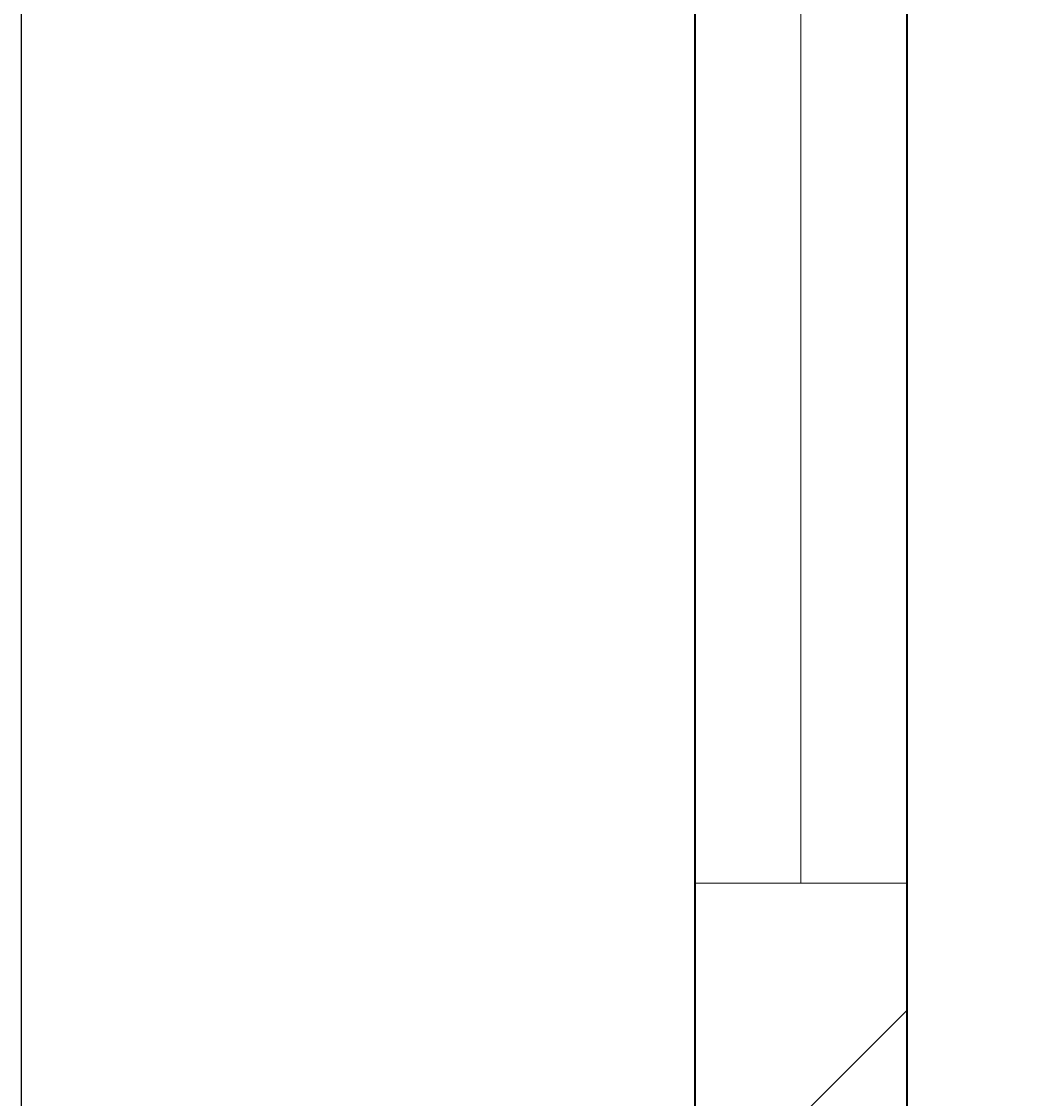
# Model space of a CAD drawing. Units: inches. Extents: x 1962 to 2771, y 1245 to 2660.
# Tile 42 of 114: x 2072.02 to 2093.47, y 2075.47 to 2098.32. Entities that reach past the tile are written whole.
import ezdxf

# ---------------------------------------------------------------- set-up
doc = ezdxf.new("R2010")
doc.units = ezdxf.units.IN
for name, color, linetype, lineweight in [('A-ANNO-DIMS', 2, 'Continuous', 18), ('A-GLAZ', 4, 'Continuous', 18), ('A-WALL', 7, 'Continuous', 35), ('A-WALL-PATT', 252, 'Continuous', 13)]:
    doc.layers.add(name, color=color, linetype=linetype, lineweight=lineweight)
doc.styles.get("Standard").update_dxf_attribs({"font": 'arial.ttf'})
doc.dimstyles.get("Standard").update_dxf_attribs({"dimtxt": 0.18, "dimasz": 0.18, "dimexe": 0.18, "dimexo": 0.0625, "dimgap": 0.09, "dimtad": 0, "dimtih": 1, "dimtoh": 1, "dimdec": 4, "dimzin": 0, "dimdsep": 46, "dimtxsty": 'Standard', "dimcen": 0.09, "dimadec": 0, "dimazin": 0, "dimtfac": 1, "dimtdec": 4, "dimtofl": 0, "dimtmove": 0, "dimatfit": 3, "dimfxl": 1, "dimtolj": 1, "dimtzin": 0, "dimarcsym": 0})

# ---------------------------------------------------------------- blocks, each defined once
blk = doc.blocks.new('WIN-60IN-A')
for p, q in [((2.25, 60), (2.25, 0)), ((2.25, 0), (0, 0)), ((0, 0), (4.5, 0))]:
    blk.add_line(p, q)
blk = doc.blocks.new('*D40')
at = {"layer": 'A-ANNO-DIMS', "color": 0, "lineweight": -2, "transparency": 16777216}
for p, q in [((2072.02, 2033.906), (2072.02, 2583.474)), ((2660.807, 2524.406), (2660.807, 2583.474)), ((2072.2, 2583.294), (2366.02, 2583.294)), ((2660.627, 2583.294), (2366.808, 2583.294))]:
    blk.add_line(p, q, dxfattribs=at)
at = {"layer": 'A-ANNO-DIMS', "color": 0, "transparency": 16777216}
for points in [[(2072.2, 2583.324), (2072.2, 2583.264), (2072.02, 2583.294)], [(2660.627, 2583.324), (2660.627, 2583.264), (2660.807, 2583.294)]]:
    blk.add_solid(points, dxfattribs=at)
at = {"layer": 'Defpoints', "color": 0, "transparency": 16777216}
for p in [(2660.807, 2583.294), (2660.807, 2524.344), (2072.02, 2033.844)]:
    blk.add_point(p, dxfattribs=at)
at = {"layer": 'A-ANNO-DIMS', "color": 0, "transparency": 16777216, "insert": (2366.414, 2583.294), "char_height": 0.18, "attachment_point": 5}
blk.add_mtext('\\A1;588.8', dxfattribs=at)
blk = doc.blocks.new('*D43')
at = {"layer": 'A-ANNO-DIMS', "color": 0, "lineweight": -2, "transparency": 16777216}
for p, q in [((2086.245, 2524.344), (2012.89, 2524.344)), ((2013.07, 2524.164), (2013.07, 2279.276)), ((2013.07, 2034.024), (2013.07, 2278.912)), ((2071.958, 2033.844), (2012.89, 2033.844))]:
    blk.add_line(p, q, dxfattribs=at)
at = {"layer": 'A-ANNO-DIMS', "color": 0, "transparency": 16777216}
for points in [[(2013.04, 2524.164), (2013.1, 2524.164), (2013.07, 2524.344)], [(2013.04, 2034.024), (2013.1, 2034.024), (2013.07, 2033.844)]]:
    blk.add_solid(points, dxfattribs=at)
at = {"layer": 'Defpoints', "color": 0, "transparency": 16777216}
for p in [(2086.307, 2524.344), (2013.07, 2033.844), (2072.02, 2033.844)]:
    blk.add_point(p, dxfattribs=at)
at = {"layer": 'A-ANNO-DIMS', "color": 0, "transparency": 16777216, "insert": (2013.07, 2279.094), "char_height": 0.18, "attachment_point": 5}
blk.add_mtext('\\A1;490.5', dxfattribs=at)

msp = doc.modelspace()

# ---------------------------------------------------------------- hatches: boundary and pattern name
at = {"layer": 'A-WALL-PATT'}
h = msp.add_hatch(dxfattribs=at)
h.set_pattern_fill('ANSI32', color=256)
h.paths.add_polyline_path([(2090.8074, 2467.3437), (2141.6481, 2467.3437), (2141.6481, 2469.5937), (2141.6481, 2471.8437), (2086.3074, 2471.8437), (2086.3074, 2422.5333), (2090.8074, 2422.5333)])
h.paths.add_polyline_path([(2282.7664, 2471.8437), (2204.8982, 2471.8437), (2204.8982, 2467.3437), (2234.8074, 2467.3437), (2234.8074, 2311.3437), (2228.7492, 2311.3437), (2228.7492, 2306.8437), (2234.8074, 2306.8437), (2331.9227, 2306.8437), (2331.9227, 2309.0937), (2331.9227, 2311.3437), (2239.3074, 2311.3437), (2239.3074, 2467.3437), (2282.7664, 2467.3437), (2282.7664, 2469.5937)])
h.paths.add_polyline_path([(2471.4531, 2519.8437), (2552.011, 2519.8437), (2564.3996, 2519.8437), (2564.3996, 2511.1389), (2568.8996, 2511.1389), (2568.8996, 2524.3437), (2466.9531, 2524.3437), (2466.9531, 2471.8437), (2450.0749, 2471.8437), (2446.4672, 2471.8437), (2446.4672, 2467.3437), (2450.0749, 2467.3437), (2475.9988, 2467.3437), (2475.9988, 2469.5937), (2475.9988, 2471.8437), (2471.4531, 2471.8437)])
h.paths.add_polyline_path([(2575.2231, 2469.5937), (2575.2231, 2471.8437), (2568.8996, 2471.8437), (2568.8996, 2487.1389), (2564.3996, 2487.1389), (2564.3996, 2471.8437), (2556.511, 2471.8437), (2499.2904, 2471.8437), (2499.2904, 2467.3437), (2507.8074, 2467.3437), (2507.8074, 2311.3437), (2414.863, 2311.3437), (2414.863, 2306.8437), (2512.3074, 2306.8437), (2517.0114, 2306.8437), (2517.0114, 2309.0937), (2517.0114, 2311.3437), (2512.3074, 2311.3437), (2512.3074, 2467.3437), (2575.2231, 2467.3437)])
h.paths.add_polyline_path([(2660.8074, 2471.8437), (2600.9602, 2471.8437), (2600.9602, 2467.3437), (2656.3074, 2467.3437), (2656.3074, 2432.5704), (2660.8074, 2432.5704)])
h.paths.add_polyline_path([(2660.8074, 2372.5704), (2656.3074, 2372.5704), (2656.3074, 2311.3437), (2600.276, 2311.3437), (2600.276, 2309.0937), (2600.276, 2306.8437), (2656.3074, 2306.8437), (2656.3074, 2296.2593), (2660.8074, 2296.2593)])
h.paths.add_polyline_path([(2572.3074, 2306.8437), (2577.1385, 2306.8437), (2577.1385, 2311.3437), (2551.082, 2311.3437), (2551.082, 2306.8437), (2567.8074, 2306.8437), (2567.8074, 2258.8437), (2540.0574, 2258.8437), (2540.0574, 2256.5937), (2540.0574, 2254.3437), (2567.8074, 2254.3437), (2656.3074, 2254.3437), (2656.3074, 2236.9085), (2660.8074, 2236.9085), (2660.8074, 2272.2593), (2656.3074, 2272.2593), (2656.3074, 2258.8437), (2572.3074, 2258.8437)])
h.paths.add_polyline_path([(2512.3074, 2254.3437), (2518.8716, 2254.3437), (2518.8716, 2256.5937), (2518.8716, 2258.8437), (2507.8074, 2258.8437), (2507.8074, 2177.8437), (2567.8074, 2177.8437), (2567.8074, 2172.9628), (2572.3074, 2172.9628), (2572.3074, 2177.8437), (2656.3074, 2177.8437), (2656.3074, 2166.4846), (2660.8074, 2166.4846), (2660.8074, 2200.9085), (2656.3074, 2200.9085), (2656.3074, 2182.3437), (2512.3074, 2182.3437)])
h.paths.add_polyline_path([(2656.3074, 2129.8437), (2572.3074, 2129.8437), (2572.3074, 2150.3044), (2570.0574, 2150.3044), (2567.8074, 2150.3044), (2567.8074, 2129.8437), (2507.8074, 2129.8437), (2507.8074, 2116.3027), (2510.0574, 2116.3027), (2512.3074, 2116.3027), (2512.3074, 2125.3437), (2567.8074, 2125.3437), (2572.3074, 2125.3437), (2656.3074, 2125.3437)])
h.paths.add_polyline_path([(2090.8074, 2362.5333), (2086.3074, 2362.5333), (2086.3074, 2298.6242), (2090.8074, 2298.6242), (2090.8074, 2306.8437), (2174.8074, 2306.8437), (2174.8074, 2286.4178), (2179.3074, 2286.4178), (2179.3074, 2306.8437), (2192.8641, 2306.8437), (2192.8641, 2309.0937), (2192.8641, 2311.3437), (2090.8074, 2311.3437)])
h.paths.add_polyline_path([(2209.156, 2258.8437), (2179.3074, 2258.8437), (2179.3074, 2263.2236), (2177.0574, 2263.2236), (2174.8074, 2263.2236), (2174.8074, 2258.8437), (2090.8074, 2258.8437), (2090.8074, 2274.6242), (2086.3074, 2274.6242), (2086.3074, 2238.2967), (2088.5574, 2238.2967), (2090.8074, 2238.2967), (2090.8074, 2254.3437), (2209.156, 2254.3437)])
h.paths.add_polyline_path([(2090.8074, 2177.8437), (2234.8074, 2177.8437), (2234.8074, 2173.1428), (2239.3074, 2173.1428), (2239.3074, 2258.8437), (2230.8442, 2258.8437), (2230.8442, 2256.5937), (2230.8442, 2254.3437), (2234.8074, 2254.3437), (2234.8074, 2182.3437), (2090.8074, 2182.3437), (2090.8074, 2202.2967), (2086.3074, 2202.2967), (2086.3074, 2140.0389), (2090.8074, 2140.0389)])
h.paths.add_polyline_path([(2090.8074, 2080.0389), (2086.3074, 2080.0389), (2086.3074, 2033.8437), (2090.8074, 2033.8437)], flags=17)
h.paths.add_polyline_path([(2244.9405, 2033.8437), (2239.3074, 2033.8437), (2239.3074, 2142.0665), (2237.2592, 2142.0665), (2234.8074, 2142.0665), (2234.8074, 2033.8437), (2090.8074, 2033.8437), (2076.5204, 2033.8437), (2072.0204, 2033.8437), (2072.0204, 2000.4493), (2076.5204, 2000.4493), (2076.5204, 2029.3437), (2090.8074, 2029.3437), (2244.9405, 2029.3437), (2244.9405, 2031.5937)])
h.paths.add_polyline_path([(2234.8074, 1933.3437), (2076.5204, 1933.3437), (2076.5204, 1952.4493), (2074.2704, 1952.4493), (2072.0204, 1952.4493), (2072.0204, 1933.3437), (2072.0204, 1928.8437), (2234.8074, 1928.8437)])
h.paths.add_polyline_path([(2090.8074, 1928.8437), (2086.3074, 1928.8437), (2086.3074, 1906.5013), (2090.8074, 1906.5013)])
h.paths.add_polyline_path([(2090.8074, 1846.5013), (2086.3074, 1846.5013), (2086.3074, 1769.9917), (2088.5574, 1769.9917), (2090.8074, 1769.9917), (2090.8074, 1780.3437), (2234.8074, 1780.3437), (2234.8074, 1708.3437), (2230.3764, 1708.3437), (2230.3764, 1703.8437), (2239.3074, 1703.8437), (2239.3074, 1792.6669), (2237.0574, 1792.6669), (2234.8074, 1792.6669), (2234.8074, 1784.8437), (2090.8074, 1784.8437)])
h.paths.add_polyline_path([(2239.3074, 1928.8437), (2244.9405, 1928.8437), (2244.9405, 1931.0937), (2244.9405, 1933.3437), (2234.8074, 1933.3437), (2234.8074, 1928.8437), (2234.8074, 1825.5949), (2239.3074, 1825.5949)])
h.paths.add_polyline_path([(2148.0425, 1649.0937), (2148.0425, 1651.3437), (2090.8074, 1651.3437), (2090.8074, 1646.8437), (2148.0425, 1646.8437)], flags=0)
h.paths.add_polyline_path([(2207.5601, 1708.3437), (2090.8074, 1708.3437), (2090.8074, 1703.8437), (2174.8074, 1703.8437), (2174.8074, 1651.3437), (2170.4457, 1651.3437), (2170.4457, 1646.8437), (2195.9924, 1646.8437), (2195.9924, 1649.0937), (2195.9924, 1651.3437), (2179.3074, 1651.3437), (2179.3074, 1703.8437), (2207.5601, 1703.8437), (2207.5601, 1706.0937)])
h.paths.add_polyline_path([(2090.8074, 1733.9917), (2086.3074, 1733.9917), (2086.3074, 1696.1032), (2088.5574, 1696.1032), (2090.8074, 1696.1032)])
h.paths.add_polyline_path([(2090.8074, 1672.1032), (2086.3074, 1672.1032), (2086.3074, 1600.3335), (2090.8074, 1600.3335)])
h.paths.add_polyline_path([(2090.8074, 1540.3335), (2086.3074, 1540.3335), (2086.3074, 1486.3437), (2139.6766, 1486.3437), (2139.6766, 1490.8437), (2090.8074, 1490.8437)])
h.paths.add_polyline_path([(2302.3876, 1490.8437), (2239.3074, 1490.8437), (2239.3074, 1646.8437), (2335.9994, 1646.8437), (2335.9994, 1651.3437), (2229.884, 1651.3437), (2229.884, 1646.8437), (2234.8074, 1646.8437), (2234.8074, 1490.8437), (2202.7103, 1490.8437), (2202.7103, 1488.5937), (2202.7103, 1486.3437), (2275.0699, 1486.3437), (2275.0699, 1475.772), (2279.5699, 1475.772), (2279.5699, 1486.3437), (2302.3876, 1486.3437)])
h.paths.add_polyline_path([(2279.5699, 1451.772), (2275.0699, 1451.772), (2275.0699, 1438.3437), (2174.8074, 1438.3437), (2174.8074, 1486.3437), (2179.7922, 1486.3437), (2179.7922, 1490.8437), (2163.3585, 1490.8437), (2163.3585, 1488.5937), (2163.3585, 1486.3437), (2170.3074, 1486.3437), (2170.3074, 1433.8437), (2279.5699, 1433.8437)])
h.paths.add_polyline_path([(2427.2363, 1490.8437), (2375.8074, 1490.8437), (2375.8074, 1646.8437), (2381.6401, 1646.8437), (2381.6401, 1651.3437), (2365.887, 1651.3437), (2365.887, 1649.0937), (2365.887, 1646.8437), (2371.3074, 1646.8437), (2371.3074, 1490.8437), (2327.5627, 1490.8437), (2327.5627, 1488.5937), (2327.5627, 1486.3437), (2371.3074, 1486.3437), (2371.3074, 1433.8437), (2375.8074, 1433.8437), (2375.8074, 1486.3437), (2427.2363, 1486.3437)])
h.paths.add_polyline_path([(2512.3074, 1646.8437), (2519.4351, 1646.8437), (2519.4351, 1649.0937), (2519.4351, 1651.3437), (2507.8074, 1651.3437), (2416.0063, 1651.3437), (2416.0063, 1649.0937), (2416.0063, 1646.8437), (2507.8074, 1646.8437), (2507.8074, 1490.8437), (2497.0532, 1490.8437), (2497.0532, 1488.5937), (2497.0532, 1486.3437), (2574.9344, 1486.3437), (2574.9344, 1476.0181), (2579.4344, 1476.0181), (2579.4344, 1486.3437), (2584.4872, 1486.3437), (2584.3074, 1490.8437), (2512.3074, 1490.8437)])
h.paths.add_polyline_path([(2470.5091, 1486.3437), (2473.9767, 1486.3437), (2473.9767, 1490.8437), (2449.6605, 1490.8437), (2449.6605, 1488.5937), (2449.6605, 1486.3437), (2466.0091, 1486.3437), (2466.0091, 1433.8437), (2470.5091, 1433.8437), (2579.4344, 1433.8437), (2579.4344, 1452.0181), (2574.9344, 1452.0181), (2574.9344, 1438.3437), (2554.5091, 1438.3437), (2470.5091, 1438.3437)])
h.paths.add_polyline_path([(2656.3074, 1490.8437), (2611.86, 1490.8437), (2611.86, 1486.3437), (2656.3074, 1486.3437)])
h.paths.add_polyline_path([(2660.8074, 1532.7007), (2658.5574, 1532.7007), (2656.3074, 1532.7007), (2656.3074, 1486.3437), (2660.8074, 1486.3437)])
h.paths.add_polyline_path([(2660.8074, 1664.9663), (2656.3074, 1664.9663), (2656.3074, 1651.3437), (2602.2313, 1651.3437), (2602.2313, 1646.8437), (2656.3074, 1646.8437), (2656.3074, 1592.7007), (2660.8074, 1592.7007)])
h.paths.add_polyline_path([(2660.8074, 1724.5221), (2656.3074, 1724.5221), (2656.3074, 1703.8437), (2542.4725, 1703.8437), (2542.4725, 1699.3437), (2567.8074, 1699.3437), (2567.8074, 1651.3437), (2552.7766, 1651.3437), (2552.7766, 1649.0937), (2552.7766, 1646.8437), (2577.2878, 1646.8437), (2577.2878, 1649.0937), (2577.2878, 1651.3437), (2572.3074, 1651.3437), (2572.3074, 1699.3437), (2656.3074, 1699.3437), (2656.3074, 1688.9663), (2660.8074, 1688.9663)])
h.paths.add_polyline_path([(2660.8074, 1880.6524), (2656.3074, 1880.6524), (2656.3074, 1832.8437), (2512.3074, 1832.8437), (2512.3074, 1837.8959), (2507.8074, 1837.8959), (2507.8074, 1828.3437), (2567.8074, 1828.3437), (2567.8074, 1804.3437), (2572.3074, 1804.3437), (2572.3074, 1828.3437), (2656.3074, 1828.3437), (2656.3074, 1818.6778), (2660.8074, 1818.6778)])
h.paths.add_polyline_path([(2660.8074, 1794.6778), (2656.3074, 1794.6778), (2656.3074, 1780.3437), (2572.3074, 1780.3437), (2572.3074, 1783.0303), (2570.0574, 1783.0303), (2567.8074, 1783.0303), (2567.8074, 1780.3437), (2507.8074, 1780.3437), (2507.8074, 1699.3437), (2517.8858, 1699.3437), (2517.8858, 1701.5937), (2517.8858, 1703.8437), (2512.3074, 1703.8437), (2512.3074, 1775.8437), (2656.3074, 1775.8437), (2656.3074, 1760.5221), (2660.8074, 1760.5221)])
h.paths.add_polyline_path([(2660.8074, 1981.3437), (2660.8074, 2020.2808), (2658.5574, 2020.2808), (2656.3074, 2020.2808), (2656.3074, 1981.3437), (2512.3074, 1981.3437), (2512.3074, 2086.6996), (2507.8074, 2086.6996), (2507.8074, 1981.3437), (2375.8074, 1981.3437), (2375.8074, 1986.8505), (2373.5574, 1986.8505), (2371.3074, 1986.8505), (2371.3074, 1973.2607), (2375.8074, 1973.2607), (2375.8074, 1976.8437), (2507.8074, 1976.8437), (2507.8074, 1865.4281), (2510.0574, 1865.4281), (2512.3074, 1865.4281), (2512.3074, 1976.8437), (2660.8074, 1976.8437)])
h.paths.add_polyline_path([(2375.8074, 1940.297), (2373.5574, 1940.297), (2371.3074, 1940.297), (2371.3074, 1933.3437), (2278.4434, 1933.3437), (2278.4434, 1928.8437), (2371.3074, 1928.8437), (2371.3074, 1651.3437), (2375.8074, 1651.3437)])
h.paths.add_polyline_path([(2660.8074, 1976.8437), (2656.3074, 1976.8437), (2656.3074, 1940.6524), (2660.8074, 1940.6524)], flags=17)
h.paths.add_polyline_path([(2660.8074, 2142.4846), (2656.3074, 2142.4846), (2656.3074, 2080.2808), (2660.8074, 2080.2808)])
h.paths.add_polyline_path([(2381.4189, 2311.3437), (2375.8074, 2311.3437), (2375.8074, 2467.3437), (2424.7242, 2467.3437), (2424.7242, 2469.5937), (2424.7242, 2471.8437), (2375.8074, 2471.8437), (2375.8074, 2524.3437), (2371.3074, 2524.3437), (2371.3074, 2471.8437), (2307.2097, 2471.8437), (2307.2097, 2467.3437), (2371.3074, 2467.3437), (2371.3074, 2311.3437), (2366.8901, 2311.3437), (2366.8901, 2306.8437), (2371.3074, 2306.8437), (2371.3074, 2033.8437), (2279.6589, 2033.8437), (2279.6589, 2029.3437), (2371.3074, 2029.3437), (2371.3074, 2014.2598), (2375.8074, 2014.2598), (2375.8074, 2306.8437), (2381.4189, 2306.8437)])
h.paths.add_polyline_path([(2263.3074, 2524.3437), (2170.3074, 2524.3437), (2170.3074, 2519.8437), (2170.3074, 2471.8437), (2165.0312, 2471.8437), (2165.0312, 2467.3437), (2179.6721, 2467.3437), (2179.6721, 2469.5161), (2179.6721, 2471.8437), (2174.8074, 2471.8437), (2174.8074, 2519.8437), (2258.8074, 2519.8437), (2258.8074, 2511.6436), (2263.3074, 2511.6436)])
h.paths.add_polyline_path([(2245.0232, 1361.4123), (2492.9468, 1361.4123), (2492.9468, 1398.505), (2245.0232, 1398.505)], flags=9)
h.paths.add_polyline_path([(2388.1434, 2086.6936), (2425.0704, 2086.6936), (2425.0704, 2105.3509), (2388.1434, 2105.3509)], flags=9)
h.paths.add_polyline_path([(2404.922, 2242.6744), (2445.7337, 2242.6744), (2445.7337, 2261.3318), (2404.922, 2261.3318)], flags=9)
h.paths.add_polyline_path([(2269.4107, 2156.7935), (2306.3378, 2156.7935), (2306.3378, 2175.4508), (2269.4107, 2175.4508)], flags=9)
h.paths.add_polyline_path([(2269.3277, 2233.4343), (2306.2547, 2233.4343), (2306.2547, 2252.0917), (2269.3277, 2252.0917)], flags=9)
h.paths.add_polyline_path([(2431.6052, 2320.6922), (2470.4456, 2320.6922), (2470.4456, 2339.3495), (2431.6052, 2339.3495)], flags=25)
h.paths.add_polyline_path([(2249.6902, 2315.7608), (2288.5306, 2315.7608), (2288.5306, 2334.4182), (2249.6902, 2334.4182)], flags=25)
h.paths.add_polyline_path([(2096.9301, 2314.3181), (2135.7704, 2314.3181), (2135.7704, 2332.9755), (2096.9301, 2332.9755)], flags=25)
h.paths.add_polyline_path([(2134.3475, 2285.7089), (2161.4655, 2285.7089), (2161.4655, 2304.3662), (2134.3475, 2304.3662)], flags=9)
h.paths.add_polyline_path([(2126.5155, 2209.4076), (2159.9227, 2209.4076), (2159.9227, 2228.065), (2126.5155, 2228.065)], flags=25)
h.paths.add_polyline_path([(2110.5753, 2141.5299), (2149.4157, 2141.5299), (2149.4157, 2160.1872), (2110.5753, 2160.1872)], flags=25)
h.paths.add_polyline_path([(2249.8618, 1968.3317), (2286.3966, 1968.3317), (2286.3966, 1986.989), (2249.8618, 1986.989)], flags=9)
h.paths.add_polyline_path([(2395.9507, 1777.0051), (2436.7624, 1777.0051), (2436.7624, 1795.6625), (2395.9507, 1795.6625)], flags=9)
h.paths.add_polyline_path([(2398.5259, 1888.5651), (2435.0062, 1888.5651), (2435.0062, 1907.2224), (2398.5259, 1907.2224)], flags=25)
h.paths.add_polyline_path([(2259.3506, 1728.3559), (2296.2776, 1728.3559), (2296.2776, 1747.0132), (2259.3506, 1747.0132)], flags=9)
h.paths.add_polyline_path([(2271.3698, 1845.268), (2308.2968, 1845.268), (2308.2968, 1863.9253), (2271.3698, 1863.9253)], flags=9)
h.paths.add_polyline_path([(2120.9355, 1786.3027), (2159.7759, 1786.3027), (2159.7759, 1804.9601), (2120.9355, 1804.9601)], flags=25)
h.paths.add_polyline_path([(2121.3164, 1732.1043), (2154.7236, 1732.1043), (2154.7236, 1750.7616), (2121.3164, 1750.7616)], flags=25)
h.paths.add_polyline_path([(2118.3706, 1678.8997), (2147.5282, 1678.8997), (2147.5282, 1697.557), (2118.3706, 1697.557)], flags=25)
h.paths.add_polyline_path([(2385.9227, 1493.557), (2424.763, 1493.557), (2424.763, 1512.2143), (2385.9227, 1512.2143)], flags=25)
h.paths.add_polyline_path([(2248.7058, 1500.0256), (2287.5462, 1500.0256), (2287.5462, 1518.6829), (2248.7058, 1518.6829)], flags=25)
h.paths.add_polyline_path([(2104.1669, 1617.3771), (2143.0073, 1617.3771), (2143.0073, 1636.0344), (2104.1669, 1636.0344)], flags=9)
h.paths.add_polyline_path([(2096.0714, 1447.8824), (2137.3845, 1447.8824), (2137.3845, 1458.1859), (2096.0714, 1458.1859)], flags=9)
h.paths.add_polyline_path([(2180.6114, 1440.325), (2209.7689, 1440.325), (2209.7689, 1458.9823), (2180.6114, 1458.9823)], flags=25)
h.paths.add_polyline_path([(2316.1698, 1447.9637), (2357.4829, 1447.9637), (2357.4829, 1458.2673), (2316.1698, 1458.2673)], flags=9)
h.paths.add_polyline_path([(2397.6187, 1447.9637), (2438.9318, 1447.9637), (2438.9318, 1458.2673), (2397.6187, 1458.2673)], flags=9)
h.paths.add_polyline_path([(2473.0778, 1439.5953), (2502.2354, 1439.5953), (2502.2354, 1458.2527), (2473.0778, 1458.2527)], flags=25)
h.paths.add_polyline_path([(2589.7027, 1447.8819), (2631.0158, 1447.8819), (2631.0158, 1458.1855), (2589.7027, 1458.1855)], flags=9)
h.paths.add_polyline_path([(2522.4009, 1497.5285), (2561.2413, 1497.5285), (2561.2413, 1516.1859), (2522.4009, 1516.1859)], flags=25)
h.paths.add_polyline_path([(2579.6565, 1671.3482), (2608.8141, 1671.3482), (2608.8141, 1690.0056), (2579.6565, 1690.0056)], flags=25)
h.paths.add_polyline_path([(2544.7038, 1725.5064), (2578.1111, 1725.5064), (2578.1111, 1744.1637), (2544.7038, 1744.1637)], flags=25)
h.paths.add_polyline_path([(2578.1191, 1807.472), (2607.2766, 1807.472), (2607.2766, 1826.1293), (2578.1191, 1826.1293)], flags=25)
h.paths.add_polyline_path([(2595.0614, 1835.1839), (2633.9018, 1835.1839), (2633.9018, 1853.8413), (2595.0614, 1853.8413)], flags=25)
h.paths.add_polyline_path([(2567.0097, 2097.7035), (2605.8501, 2097.7035), (2605.8501, 2116.3609), (2567.0097, 2116.3609)], flags=9)
h.paths.add_polyline_path([(2586.644, 2134.6454), (2615.8015, 2134.6454), (2615.8015, 2153.3027), (2586.644, 2153.3027)], flags=9)
h.paths.add_polyline_path([(2544.6185, 2212.6783), (2578.0258, 2212.6783), (2578.0258, 2231.3356), (2544.6185, 2231.3356)], flags=25)
h.paths.add_polyline_path([(2577.0273, 2256.9023), (2606.1849, 2256.9023), (2606.1849, 2275.5597), (2577.0273, 2275.5597)], flags=24)
h.paths.add_polyline_path([(2605.2683, 2315.2821), (2644.1087, 2315.2821), (2644.1087, 2333.9395), (2605.2683, 2333.9395)], flags=25)
h.paths.add_polyline_path([(2583.1244, 2496.1815), (2624.4375, 2496.1815), (2624.4375, 2506.4851), (2583.1244, 2506.4851)], flags=9)
h.paths.add_polyline_path([(2474.761, 2497.0823), (2503.9185, 2497.0823), (2503.9185, 2515.7397), (2474.761, 2515.7397)], flags=25)
h.paths.add_polyline_path([(2387.5787, 2494.2563), (2428.902, 2494.2563), (2428.902, 2504.5598), (2387.5787, 2504.5598)], flags=9)
h.paths.add_polyline_path([(2300.1657, 2500.1564), (2341.4788, 2500.1564), (2341.4788, 2510.46), (2300.1657, 2510.46)], flags=25)
h.paths.add_polyline_path([(2176.8589, 2497.5843), (2206.0165, 2497.5843), (2206.0165, 2516.2416), (2176.8589, 2516.2416)], flags=25)
h.paths.add_polyline_path([(2097.4668, 2494.9762), (2138.7799, 2494.9762), (2138.7799, 2505.2798), (2097.4668, 2505.2798)], flags=9)

# ---------------------------------------------------------------- linework, layer by layer
at = {"layer": 'A-WALL'}
for p, q in [((2086.3074, 2471.8437), (2086.3074, 2033.8437)), ((2090.8074, 2177.8437), (2090.8074, 2033.8437))]:
    msp.add_line(p, q, dxfattribs=at)

# ---------------------------------------------------------------- block references
at = {"layer": 'A-GLAZ'}
msp.add_blockref('WIN-60IN-A', (2086.3074, 2080.0389), dxfattribs=at)

# ---------------------------------------------------------------- dimensions: what is measured, and where the dimension line sits
at = {"layer": 'A-ANNO-DIMS'}
dim = msp.add_linear_dim(base=(2660.8074, 2583.2937), p1=(2072.0204, 2033.8437), p2=(2660.8074, 2524.3437), dimstyle='Standard', override={"dimdec": 1, "dimlfac": 1, "dimrnd": 0, "dimzin": 0, "dimdsep": 46, "dimlunit": 2}, dxfattribs=at)
dim.commit()
dim.dimension.update_dxf_attribs({"geometry": '*D40', "text_midpoint": (2366.4139, 2583.2937)})
dim = msp.add_linear_dim(base=(2013.0704, 2033.8437), p1=(2086.3074, 2524.3437), p2=(2072.0204, 2033.8437), angle=90, dimstyle='Standard', override={"dimdec": 1, "dimlfac": 1, "dimrnd": 0, "dimzin": 0, "dimdsep": 46, "dimlunit": 2}, dxfattribs=at)
dim.commit()
dim.dimension.update_dxf_attribs({"geometry": '*D43', "text_midpoint": (2013.0704, 2279.0937)})

doc.saveas('drawing.dxf')
